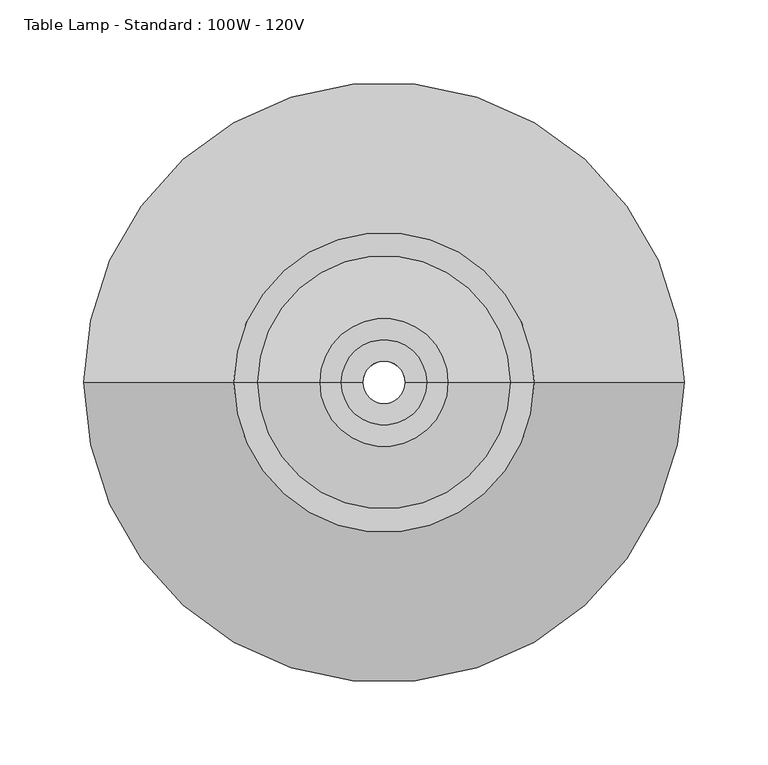
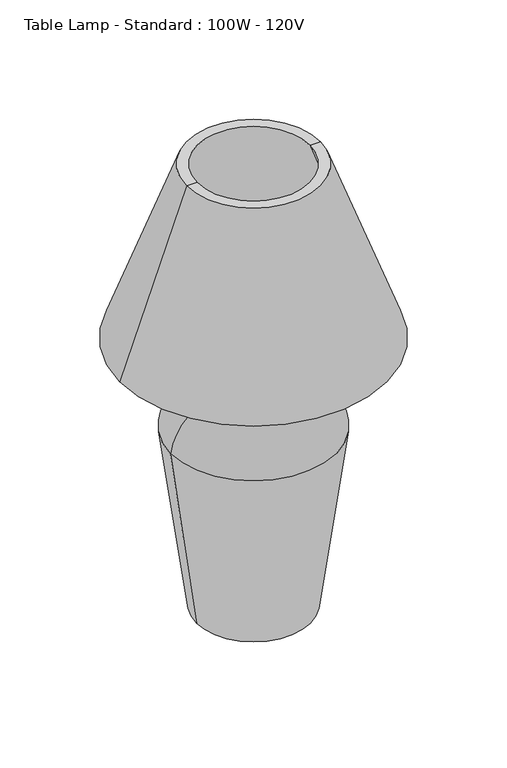
"""IFC4 building model written with IfcOpenShell, lengths in millimetres: light fixture geometry, Table Lamp - Standard : 100W - 120V."""

from ifc_helpers import new_model, si_unit, point, frame, origin, origin_with_axes, place, context, project, spatial, polyline, circle_curve, ellipse_curve, trimmed, source, transform, mapped, element, save
from ifc_brep_helpers import plane_surface, cylinder_surface, revolved_surface, advanced_brep


def table_lamp_standard_100w_120v_6e8cd8b1(model_context):
    return source(origin(), model_context, "Body", "AdvancedBrep", [
        advanced_brep(
        [(-164.7317588, 0.0, 376.8232721), (164.7317588, 0.0, 376.8232721), (75.4334235, 0.0, 622.168432), (-75.4334235, 0.0, 622.168432), (-178.6712043, 0.0, 376.8232721), (178.6712043, 0.0, 376.8232721), (-89.372869, 0.0, 622.168432), (89.372869, 0.0, 622.168432)],
        [
            (0, 1, circle_curve(frame((0.0, 0.0, 376.8232721), z_axis=(0.0, 0.0, -1.0), x_axis=(1.0, 0.0, 0.0)), 164.7317588)),
            (1, 2),
            (2, 3, circle_curve(frame((0.0, 0.0, 622.168432), z_axis=(0.0, 0.0, 1.0), x_axis=(1.0, 0.0, 0.0)), 75.4334235)),
            (3, 0),
            (1, 0, circle_curve(frame((0.0, 0.0, 376.8232721), z_axis=(0.0, 0.0, -1.0), x_axis=(1.0, 0.0, 0.0)), 164.7317588)),
            (3, 2, circle_curve(frame((0.0, 0.0, 622.168432), z_axis=(0.0, 0.0, 1.0), x_axis=(1.0, 0.0, 0.0)), 75.4334235)),
            (4, 5, circle_curve(frame((0.0, 0.0, 376.8232721), z_axis=(0.0, 0.0, -1.0), x_axis=(1.0, 0.0, 0.0)), 178.6712043)),
            (5, 1),
            (0, 4),
            (5, 4, circle_curve(frame((0.0, 0.0, 376.8232721), z_axis=(0.0, 0.0, -1.0), x_axis=(1.0, 0.0, 0.0)), 178.6712043)),
            (6, 7, circle_curve(frame((0.0, 0.0, 622.168432), z_axis=(0.0, 0.0, -1.0), x_axis=(1.0, 0.0, 0.0)), 89.372869)),
            (7, 5),
            (4, 6),
            (7, 6, circle_curve(frame((0.0, 0.0, 622.168432), z_axis=(0.0, 0.0, -1.0), x_axis=(1.0, 0.0, 0.0)), 89.372869)),
            (2, 7),
            (6, 3),
        ],
        [
            revolved_surface(polyline([(75.4334235, 0.0, 622.168432), (164.7317588, 0.0, 376.8232721)]), (0.0, 0.0, 736.6), (0.0, 0.0, 1.0)),
            plane_surface(frame((0.0, 0.0, 376.8232721), z_axis=(0.0, 0.0, -1.0), x_axis=(1.0, 0.0, 0.0))),
            revolved_surface(polyline([(178.6712043, 0.0, 376.8232721), (89.372869, 0.0, 622.168432)]), (0.0, 0.0, 736.6), (0.0, 0.0, 1.0)),
            plane_surface(frame((0.0, 0.0, 622.168432), z_axis=(0.0, 0.0, 1.0), x_axis=(1.0, 0.0, 0.0))),
        ],
        [
            (0, [[1, 2, 3, 4]]),
            (0, [[5, -4, 6, -2]]),
            (1, [[7, 8, -1, 9]]),
            (1, [[10, -9, -5, -8]]),
            (2, [[11, 12, -7, 13]]),
            (2, [[14, -13, -10, -12]]),
            (3, [[-3, 15, -11, 16]]),
            (3, [[-6, -16, -14, -15]]),
        ],
    ),
        advanced_brep(
        [(-25.4, 0.0, 363.9152112), (25.4, 0.0, 363.9152112), (25.4, 0.0, 338.5152112), (-25.4, 0.0, 338.5152112), (-12.7, 0.0, 363.9152112), (12.7, 0.0, 363.9152112), (-12.7, 0.0, 338.5152112), (12.7, 0.0, 338.5152112)],
        [
            (0, 1, circle_curve(frame((0.0, 0.0, 363.9152112), z_axis=(0.0, 0.0, -1.0), x_axis=(1.0, 0.0, 0.0)), 25.4)),
            (1, 2),
            (2, 3, circle_curve(frame((0.0, 0.0, 338.5152112), z_axis=(0.0, 0.0, 1.0), x_axis=(1.0, 0.0, 0.0)), 25.4)),
            (3, 0),
            (1, 0, circle_curve(frame((0.0, 0.0, 363.9152112), z_axis=(0.0, 0.0, -1.0), x_axis=(1.0, 0.0, 0.0)), 25.4)),
            (3, 2, circle_curve(frame((0.0, 0.0, 338.5152112), z_axis=(0.0, 0.0, 1.0), x_axis=(1.0, 0.0, 0.0)), 25.4)),
            (4, 5, circle_curve(frame((0.0, 0.0, 363.9152112), z_axis=(0.0, 0.0, -1.0), x_axis=(1.0, 0.0, 0.0)), 12.7)),
            (5, 1),
            (0, 4),
            (5, 4, circle_curve(frame((0.0, 0.0, 363.9152112), z_axis=(0.0, 0.0, -1.0), x_axis=(1.0, 0.0, 0.0)), 12.7)),
            (6, 7, circle_curve(frame((0.0, 0.0, 338.5152112), z_axis=(0.0, 0.0, -1.0), x_axis=(1.0, 0.0, 0.0)), 12.7)),
            (7, 5),
            (4, 6),
            (7, 6, circle_curve(frame((0.0, 0.0, 338.5152112), z_axis=(0.0, 0.0, -1.0), x_axis=(1.0, 0.0, 0.0)), 12.7)),
            (2, 7),
            (6, 3),
        ],
        [
            cylinder_surface(frame((0.0, 0.0, 457.2), z_axis=(0.0, 0.0, 1.0), x_axis=(1.0, 0.0, 0.0)), 25.4),
            plane_surface(frame((0.0, 0.0, 363.9152112), z_axis=(0.0, 0.0, 1.0), x_axis=(1.0, 0.0, 0.0))),
            revolved_surface(polyline([(12.7, 0.0, 363.9152112), (12.7, 0.0, 338.5152112)]), (0.0, 0.0, 457.2), (0.0, 0.0, 1.0)),
            plane_surface(frame((0.0, 0.0, 338.5152112), z_axis=(0.0, 0.0, -1.0), x_axis=(1.0, 0.0, 0.0))),
        ],
        [
            (0, [[1, 2, 3, 4]]),
            (0, [[5, -4, 6, -2]]),
            (1, [[7, 8, -1, 9]]),
            (1, [[10, -9, -5, -8]]),
            (2, [[11, 12, -7, 13]]),
            (2, [[14, -13, -10, -12]]),
            (3, [[-3, 15, -11, 16]]),
            (3, [[-6, -16, -14, -15]]),
        ],
    ),
        advanced_brep(
        [(-38.1, 0.0, 300.4152112), (38.1, 0.0, 300.4152112), (12.7, 0.0, 300.4152112), (-12.7, 0.0, 300.4152112), (-38.1, 0.0, 338.5152112), (38.1, 0.0, 338.5152112), (-12.7, 0.0, 338.5152112), (12.7, 0.0, 338.5152112)],
        [
            (0, 1, circle_curve(frame((0.0, 0.0, 300.4152112), z_axis=(0.0, 0.0, -1.0), x_axis=(1.0, 0.0, 0.0)), 38.1)),
            (1, 2),
            (2, 3, circle_curve(frame((0.0, 0.0, 300.4152112), z_axis=(0.0, 0.0, 1.0), x_axis=(1.0, 0.0, 0.0)), 12.7)),
            (3, 0),
            (1, 0, circle_curve(frame((0.0, 0.0, 300.4152112), z_axis=(0.0, 0.0, -1.0), x_axis=(1.0, 0.0, 0.0)), 38.1)),
            (3, 2, circle_curve(frame((0.0, 0.0, 300.4152112), z_axis=(0.0, 0.0, 1.0), x_axis=(1.0, 0.0, 0.0)), 12.7)),
            (4, 5, circle_curve(frame((0.0, 0.0, 338.5152112), z_axis=(0.0, 0.0, -1.0), x_axis=(1.0, 0.0, 0.0)), 38.1)),
            (5, 1),
            (0, 4),
            (5, 4, circle_curve(frame((0.0, 0.0, 338.5152112), z_axis=(0.0, 0.0, -1.0), x_axis=(1.0, 0.0, 0.0)), 38.1)),
            (6, 7, circle_curve(frame((0.0, 0.0, 338.5152112), z_axis=(0.0, 0.0, -1.0), x_axis=(1.0, 0.0, 0.0)), 12.7)),
            (7, 5),
            (4, 6),
            (7, 6, circle_curve(frame((0.0, 0.0, 338.5152112), z_axis=(0.0, 0.0, -1.0), x_axis=(1.0, 0.0, 0.0)), 12.7)),
            (2, 7),
            (6, 3),
        ],
        [
            plane_surface(frame((0.0, 0.0, 300.4152112), z_axis=(0.0, 0.0, -1.0), x_axis=(1.0, 0.0, 0.0))),
            cylinder_surface(frame((0.0, 0.0, 431.8), z_axis=(0.0, 0.0, 1.0), x_axis=(1.0, 0.0, 0.0)), 38.1),
            plane_surface(frame((0.0, 0.0, 338.5152112), z_axis=(0.0, 0.0, 1.0), x_axis=(1.0, 0.0, 0.0))),
            revolved_surface(polyline([(12.7, 0.0, 338.5152112), (12.7, 0.0, 300.4152112)]), (0.0, 0.0, 431.8), (0.0, 0.0, 1.0)),
        ],
        [
            (0, [[1, 2, 3, 4]]),
            (0, [[5, -4, 6, -2]]),
            (1, [[7, 8, -1, 9]]),
            (1, [[10, -9, -5, -8]]),
            (2, [[11, 12, -7, 13]]),
            (2, [[14, -13, -10, -12]]),
            (3, [[-3, 15, -11, 16]]),
            (3, [[-6, -16, -14, -15]]),
        ],
    ),
        advanced_brep(
        [(-110.728718, 0.0, 251.659832), (110.728718, 0.0, 251.659832), (76.2, 0.0, 0.0), (-76.2, 0.0, 0.0), (-38.1, 0.0, 310.9616106), (38.1, 0.0, 310.9616106), (-38.1, 0.0, 300.4152112), (38.1, 0.0, 300.4152112), (-98.1869356, 0.0, 253.725236), (98.1869356, 0.0, 253.725236), (-65.5434347, 0.0, 12.7), (65.5434347, 0.0, 12.7), (-12.7, 0.0, 12.7), (12.7, 0.0, 12.7), (-12.7, 0.0, 0.0), (12.7, 0.0, 0.0)],
        [
            (0, 1, circle_curve(frame((0.0, 0.0, 251.659832), z_axis=(0.0, 0.0, -1.0), x_axis=(1.0, 0.0, 0.0)), 110.728718)),
            (1, 2),
            (2, 3, circle_curve(origin_with_axes(), 76.2)),
            (3, 0),
            (1, 0, circle_curve(frame((0.0, 0.0, 251.659832), z_axis=(0.0, 0.0, -1.0), x_axis=(1.0, 0.0, 0.0)), 110.728718)),
            (3, 2, circle_curve(origin_with_axes(), 76.2)),
            (4, 5, circle_curve(frame((0.0, 0.0, 310.9616106), z_axis=(0.0, 0.0, -1.0), x_axis=(1.0, 0.0, 0.0)), 38.1)),
            (5, 1, circle_curve(frame((44.5301031, 0.0, 244.710551), z_axis=(0.0, 1.0, 0.0), x_axis=(1.0, 0.0, 0.0)), 66.5623702)),
            (0, 4, circle_curve(frame((-44.5301031, 0.0, 244.710551), z_axis=(0.0, 1.0, 0.0), x_axis=(-1.0, 0.0, 0.0)), 66.5623702)),
            (5, 4, circle_curve(frame((0.0, 0.0, 310.9616106), z_axis=(0.0, 0.0, -1.0), x_axis=(1.0, 0.0, 0.0)), 38.1)),
            (6, 7, circle_curve(frame((0.0, 0.0, 300.4152112), z_axis=(0.0, 0.0, -1.0), x_axis=(1.0, 0.0, 0.0)), 38.1)),
            (7, 5),
            (4, 6),
            (7, 6, circle_curve(frame((0.0, 0.0, 300.4152112), z_axis=(0.0, 0.0, -1.0), x_axis=(1.0, 0.0, 0.0)), 38.1)),
            (8, 9, circle_curve(frame((0.0, 0.0, 253.725236), z_axis=(0.0, 0.0, -1.0), x_axis=(1.0, 0.0, 0.0)), 98.1869356)),
            (9, 7, circle_curve(frame((44.5301031, 0.0, 246.6813721), z_axis=(0.0, -1.0, 0.0), x_axis=(1.0, 0.0, 0.0)), 54.1172033)),
            (6, 8, circle_curve(frame((-44.5301031, 0.0, 246.6813721), z_axis=(0.0, -1.0, 0.0), x_axis=(-1.0, 0.0, 0.0)), 54.1172033)),
            (9, 8, circle_curve(frame((0.0, 0.0, 253.725236), z_axis=(0.0, 0.0, -1.0), x_axis=(1.0, 0.0, 0.0)), 98.1869356)),
            (10, 11, circle_curve(frame((0.0, 0.0, 12.7), z_axis=(0.0, 0.0, -1.0), x_axis=(1.0, 0.0, 0.0)), 65.5434347)),
            (11, 9),
            (8, 10),
            (11, 10, circle_curve(frame((0.0, 0.0, 12.7), z_axis=(0.0, 0.0, -1.0), x_axis=(1.0, 0.0, 0.0)), 65.5434347)),
            (12, 13, circle_curve(frame((0.0, 0.0, 12.7), z_axis=(0.0, 0.0, -1.0), x_axis=(1.0, 0.0, 0.0)), 12.7)),
            (13, 11),
            (10, 12),
            (13, 12, circle_curve(frame((0.0, 0.0, 12.7), z_axis=(0.0, 0.0, -1.0), x_axis=(1.0, 0.0, 0.0)), 12.7)),
            (14, 15, circle_curve(frame((0.0, 0.0, 0.0), z_axis=(0.0, 0.0, -1.0), x_axis=(1.0, 0.0, 0.0)), 12.7)),
            (15, 13),
            (12, 14),
            (15, 14, circle_curve(frame((0.0, 0.0, 0.0), z_axis=(0.0, 0.0, -1.0), x_axis=(1.0, 0.0, 0.0)), 12.7)),
            (2, 15),
            (14, 3),
        ],
        [
            revolved_surface(polyline([(76.2, 0.0, 0.0), (110.728718, 0.0, 251.659832)]), (0.0, 0.0, -50.8), (0.0, 0.0, 1.0)),
            revolved_surface(trimmed(ellipse_curve(frame((44.5301031, 0.0, 244.710551), z_axis=(0.0, -1.0, 0.0), x_axis=(1.0, 0.0, 0.0)), 66.5623702, 66.5623702), [point((110.728718, 0.0, 251.659832))], [point((38.1, 0.0, 310.9616106))], True, "CARTESIAN"), (0.0, 0.0, -50.8), (0.0, 0.0, 1.0)),
            revolved_surface(polyline([(38.1, 0.0, 310.9616106), (38.1, 0.0, 300.4152112)]), (0.0, 0.0, -50.8), (0.0, 0.0, 1.0)),
            revolved_surface(trimmed(ellipse_curve(frame((44.5301031, 0.0, 246.6813721), z_axis=(0.0, 1.0, 0.0), x_axis=(1.0, 0.0, 0.0)), 54.1172033, 54.1172033), [point((38.1, 0.0, 300.4152112))], [point((98.1869356, 0.0, 253.725236))], True, "CARTESIAN"), (0.0, 0.0, -50.8), (0.0, 0.0, 1.0)),
            revolved_surface(polyline([(98.1869356, 0.0, 253.725236), (65.5434347, 0.0, 12.7)]), (0.0, 0.0, -50.8), (0.0, 0.0, 1.0)),
            plane_surface(frame((0.0, 0.0, 12.7), z_axis=(0.0, 0.0, 1.0), x_axis=(1.0, 0.0, 0.0))),
            revolved_surface(polyline([(12.7, 0.0, 12.700000000000003), (12.7, 0.0, 0.0)]), (0.0, 0.0, -50.8), (0.0, 0.0, 1.0)),
            plane_surface(frame((0.0, 0.0, 0.0), z_axis=(0.0, 0.0, -1.0), x_axis=(1.0, 0.0, 0.0))),
        ],
        [
            (0, [[1, 2, 3, 4]]),
            (0, [[5, -4, 6, -2]]),
            (1, [[7, 8, -1, 9]]),
            (1, [[10, -9, -5, -8]]),
            (2, [[11, 12, -7, 13]]),
            (2, [[14, -13, -10, -12]]),
            (3, [[15, 16, -11, 17]]),
            (3, [[18, -17, -14, -16]]),
            (4, [[19, 20, -15, 21]]),
            (4, [[22, -21, -18, -20]]),
            (5, [[23, 24, -19, 25]]),
            (5, [[26, -25, -22, -24]]),
            (6, [[27, 28, -23, 29]]),
            (6, [[30, -29, -26, -28]]),
            (7, [[-3, 31, -27, 32]]),
            (7, [[-6, -32, -30, -31]]),
        ],
    ),
    ])


if __name__ == "__main__":
    model = new_model("IFC4")
    model_context = context("Model", 3, world=origin())
    ifc_project = project(units=[si_unit("LENGTHUNIT", "METRE", prefix="MILLI")], contexts=[model_context])
    site = spatial("IfcSite", under=ifc_project)
    building = spatial("IfcBuilding", under=site)
    placement = place(None, origin())
    table_lamp_standard_100w_120v_shape = table_lamp_standard_100w_120v_6e8cd8b1(model_context)
    element("IfcLightFixture", 1, ObjectType="Table Lamp - Standard : 100W - 120V", at=placement, inside=building, context=model_context, shape_type="MappedRepresentation", body=[
        mapped(table_lamp_standard_100w_120v_shape, transform((0.0, 0.0, 0.0), x_axis=(1.0, 0.0, 0.0), y_axis=(0.0, 1.0, 0.0), z_axis=(0.0, 0.0, 1.0))),
    ])
    save(model, "model.ifc")

# Revit data of these elements
# Type "Table Lamp - Standard : 100W - 120V"
#   Assembly Code = "D5020220"
#   Lamp = "R-30"
#   Wattage = 100 W
#   built-in parameter 1150110 = 1 (stored number, unit not read)
#   built-in parameter 1114217 = 1 (stored number, unit not read)
#   built-in parameter 1150109 = 1 (stored number, unit not read)
#   built-in parameter 1150113 = 1 (stored number, unit not read)
#   built-in parameter 1150115 = 1 (stored number, unit not read)
#   built-in parameter 1150105 = 95.493 (stored number, unit not read)
#   Light Source Symbol Size = 2' - 0"
#   built-in parameter 1150112 = 1 (stored number, unit not read)
#   built-in parameter 1150114 = 1 (stored number, unit not read)
#   built-in parameter 1150107 = 2800 (stored number, unit not read)
#   built-in parameter 1150106 = 0.95493 (stored number, unit not read)
#   built-in parameter 1150104 = 1.11484 (stored number, unit not read)
#   Ballast Voltage = 120 V
#   built-in parameter 1114218 = 1 (stored number, unit not read)
#   built-in parameter 1150133 = 10 (stored number, unit not read)
#   Lumens = 1200 lm
#   Apparent Load = 100 VA
#   built-in parameter 1150134 = 4
#   built-in parameter 1150137 = 1
#   Color Filter = 16777215
#   built-in parameter 1140040 [instance default] = 1
#   Ballast Number of Poles = 1
#   Base Material = Plastic, Opaque Black
#   Shade Material = Glass, Frosted
#   Dimming Lamp Color Temperature Shift = (empty or 0)
#   Default Elevation = 0
#   Wattage Comments = ""
# Element 1 (IfcLightFixture, "Table Lamp - Standard : 100W - 120V")
#   Materials on its faces: "Plastic, Opaque Black", "Glass, Frosted"
# Materials
#   "Plastic, Opaque Black": class "Plastic", colour RGB 0 0 0, transparency 0.7, Description = "Plastic, generic, opaque black", Cost = 0
#   "Glass, Frosted": class "Glass", colour RGB 250 244 225, transparency 0.55, Description = "physical material", Cost = 0
